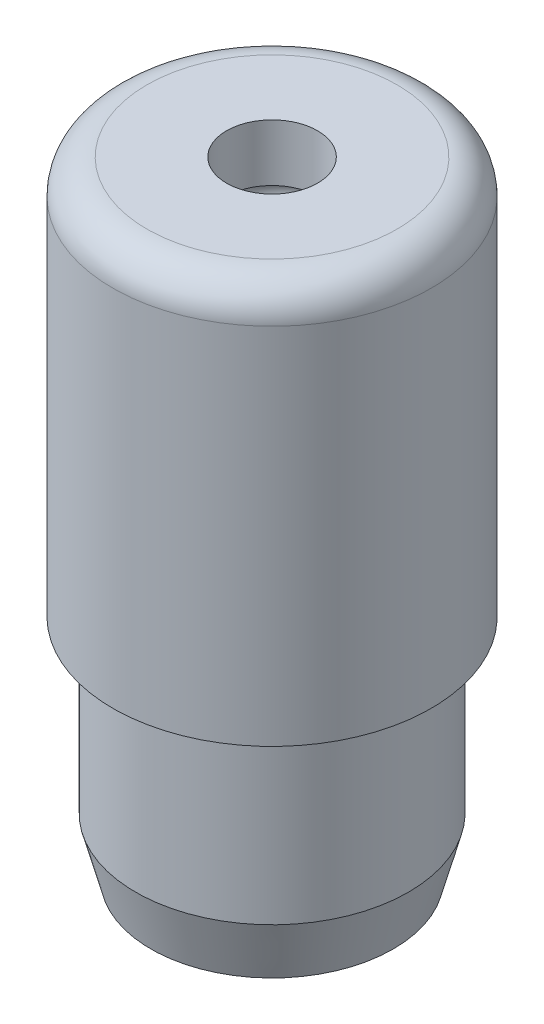
ISO-10303-21;
HEADER;
FILE_DESCRIPTION(('STEP AP214'),'2;1');
FILE_NAME('part.step','',(''),(''),'','','');
FILE_SCHEMA(('AUTOMOTIVE_DESIGN { 1 0 10303 214 1 1 1 1 }'));
ENDSEC;
DATA;
#1=APPLICATION_CONTEXT('core data for automotive mechanical design processes');
#2=APPLICATION_PROTOCOL_DEFINITION('international standard','automotive_design',2000,#1);
#3=PRODUCT_CONTEXT('',#1,'mechanical');
#4=PRODUCT('Part','Part','',(#3));
#5=PRODUCT_RELATED_PRODUCT_CATEGORY('part','',(#4));
#6=PRODUCT_DEFINITION_FORMATION('','',#4);
#7=PRODUCT_DEFINITION_CONTEXT('part definition',#1,'design');
#8=PRODUCT_DEFINITION('design','',#6,#7);
#9=PRODUCT_DEFINITION_SHAPE('','',#8);
#10=(LENGTH_UNIT() NAMED_UNIT(*) SI_UNIT(.MILLI.,.METRE.));
#11=(NAMED_UNIT(*) PLANE_ANGLE_UNIT() SI_UNIT($,.RADIAN.));
#12=(NAMED_UNIT(*) SI_UNIT($,.STERADIAN.) SOLID_ANGLE_UNIT());
#13=UNCERTAINTY_MEASURE_WITH_UNIT(LENGTH_MEASURE(1.E-05),#10,'distance_accuracy_value','');
#14=(GEOMETRIC_REPRESENTATION_CONTEXT(3) GLOBAL_UNCERTAINTY_ASSIGNED_CONTEXT((#13)) GLOBAL_UNIT_ASSIGNED_CONTEXT((#10,
#11,#12)) REPRESENTATION_CONTEXT('',''));
#15=CARTESIAN_POINT('',(0.,0.,0.));
#16=DIRECTION('',(0.,0.,1.));
#17=DIRECTION('',(1.,0.,0.));
#18=AXIS2_PLACEMENT_3D('',#15,#16,#17);
#19=CARTESIAN_POINT('',(0.,148.45149792253,0.));
#20=DIRECTION('',(0.,1.,0.));
#21=DIRECTION('',(-1.,0.,0.));
#22=AXIS2_PLACEMENT_3D('',#19,#20,#21);
#23=CYLINDRICAL_SURFACE('',#22,12.);
#24=CARTESIAN_POINT('',(0.,15.1898640484145,0.));
#25=DIRECTION('',(0.,1.,0.));
#26=DIRECTION('',(-1.,0.,0.));
#27=AXIS2_PLACEMENT_3D('',#24,#25,#26);
#28=CIRCLE('',#27,12.);
#29=CARTESIAN_POINT('',(-12.,15.1898640484145,0.));
#30=VERTEX_POINT('',#29);
#31=EDGE_CURVE('E81',#30,#30,#28,.T.);
#32=ORIENTED_EDGE('',*,*,#31,.T.);
#33=EDGE_LOOP('',(#32));
#34=FACE_BOUND('',#33,.T.);
#35=CARTESIAN_POINT('',(0.,30.1898640484145,0.));
#36=DIRECTION('',(0.,1.,0.));
#37=DIRECTION('',(-1.,0.,0.));
#38=AXIS2_PLACEMENT_3D('',#35,#36,#37);
#39=CIRCLE('',#38,12.);
#40=CARTESIAN_POINT('',(-12.,30.1898640484145,0.));
#41=VERTEX_POINT('',#40);
#42=EDGE_CURVE('E10',#41,#41,#39,.T.);
#43=ORIENTED_EDGE('',*,*,#42,.F.);
#44=EDGE_LOOP('',(#43));
#45=FACE_BOUND('',#44,.T.);
#46=ADVANCED_FACE('F40',(#34,#45),#23,.T.);
#47=CARTESIAN_POINT('',(-14.,30.1898640484145,0.));
#48=DIRECTION('',(0.,-1.,0.));
#49=DIRECTION('',(1.,0.,0.));
#50=AXIS2_PLACEMENT_3D('',#47,#48,#49);
#51=PLANE('',#50);
#52=ORIENTED_EDGE('',*,*,#42,.T.);
#53=EDGE_LOOP('',(#52));
#54=FACE_BOUND('',#53,.T.);
#55=CARTESIAN_POINT('',(0.,30.1898640484145,0.));
#56=DIRECTION('',(0.,1.,0.));
#57=DIRECTION('',(-1.,0.,0.));
#58=AXIS2_PLACEMENT_3D('',#55,#56,#57);
#59=CIRCLE('',#58,14.);
#60=CARTESIAN_POINT('',(-14.,30.1898640484145,0.));
#61=VERTEX_POINT('',#60);
#62=EDGE_CURVE('E43',#61,#61,#59,.T.);
#63=ORIENTED_EDGE('',*,*,#62,.F.);
#64=EDGE_LOOP('',(#63));
#65=FACE_BOUND('',#64,.T.);
#66=ADVANCED_FACE('F102',(#54,#65),#51,.T.);
#67=CARTESIAN_POINT('',(0.,148.45149792253,0.));
#68=DIRECTION('',(0.,1.,0.));
#69=DIRECTION('',(-1.,0.,0.));
#70=AXIS2_PLACEMENT_3D('',#67,#68,#69);
#71=CYLINDRICAL_SURFACE('',#70,14.);
#72=ORIENTED_EDGE('',*,*,#62,.T.);
#73=EDGE_LOOP('',(#72));
#74=FACE_BOUND('',#73,.T.);
#75=CARTESIAN_POINT('',(0.,62.1898640484145,0.));
#76=DIRECTION('',(0.,1.,0.));
#77=DIRECTION('',(-1.,0.,0.));
#78=AXIS2_PLACEMENT_3D('',#75,#76,#77);
#79=CIRCLE('',#78,14.);
#80=CARTESIAN_POINT('',(-14.,62.1898640484145,0.));
#81=VERTEX_POINT('',#80);
#82=EDGE_CURVE('E50',#81,#81,#79,.T.);
#83=ORIENTED_EDGE('',*,*,#82,.F.);
#84=EDGE_LOOP('',(#83));
#85=FACE_BOUND('',#84,.T.);
#86=ADVANCED_FACE('F103',(#74,#85),#71,.T.);
#87=CARTESIAN_POINT('',(0.,62.1898640484145,0.));
#88=DIRECTION('',(0.,1.,0.));
#89=DIRECTION('',(-1.,0.,0.));
#90=AXIS2_PLACEMENT_3D('',#87,#88,#89);
#91=TOROIDAL_SURFACE('',#90,11.,3.);
#92=ORIENTED_EDGE('',*,*,#82,.T.);
#93=EDGE_LOOP('',(#92));
#94=FACE_BOUND('',#93,.T.);
#95=CARTESIAN_POINT('',(0.,65.1898640484145,0.));
#96=DIRECTION('',(0.,1.,0.));
#97=DIRECTION('',(-1.,0.,0.));
#98=AXIS2_PLACEMENT_3D('',#95,#96,#97);
#99=CIRCLE('',#98,11.);
#100=CARTESIAN_POINT('',(-11.,65.1898640484145,0.));
#101=VERTEX_POINT('',#100);
#102=EDGE_CURVE('E51',#101,#101,#99,.T.);
#103=ORIENTED_EDGE('',*,*,#102,.F.);
#104=EDGE_LOOP('',(#103));
#105=FACE_BOUND('',#104,.T.);
#106=ADVANCED_FACE('F109',(#94,#105),#91,.T.);
#107=CARTESIAN_POINT('',(-4.0000000000018,65.1898640484145,0.));
#108=DIRECTION('',(0.,1.,0.));
#109=DIRECTION('',(-1.,0.,0.));
#110=AXIS2_PLACEMENT_3D('',#107,#108,#109);
#111=PLANE('',#110);
#112=ORIENTED_EDGE('',*,*,#102,.T.);
#113=EDGE_LOOP('',(#112));
#114=FACE_BOUND('',#113,.T.);
#115=CARTESIAN_POINT('',(0.,65.1898640484145,0.));
#116=DIRECTION('',(0.,1.,0.));
#117=DIRECTION('',(-1.,0.,0.));
#118=AXIS2_PLACEMENT_3D('',#115,#116,#117);
#119=CIRCLE('',#118,4.00000000000181);
#120=CARTESIAN_POINT('',(-4.0000000000018,65.1898640484145,0.));
#121=VERTEX_POINT('',#120);
#122=EDGE_CURVE('E57',#121,#121,#119,.T.);
#123=ORIENTED_EDGE('',*,*,#122,.F.);
#124=EDGE_LOOP('',(#123));
#125=FACE_BOUND('',#124,.T.);
#126=ADVANCED_FACE('F113',(#114,#125),#111,.T.);
#127=CARTESIAN_POINT('',(0.,148.45149792253,0.));
#128=DIRECTION('',(0.,1.,0.));
#129=DIRECTION('',(-1.,0.,0.));
#130=AXIS2_PLACEMENT_3D('',#127,#128,#129);
#131=CYLINDRICAL_SURFACE('',#130,4.00000000000181);
#132=ORIENTED_EDGE('',*,*,#122,.T.);
#133=EDGE_LOOP('',(#132));
#134=FACE_BOUND('',#133,.T.);
#135=CARTESIAN_POINT('',(0.,60.1898640484145,0.));
#136=DIRECTION('',(0.,1.,0.));
#137=DIRECTION('',(-1.,0.,0.));
#138=AXIS2_PLACEMENT_3D('',#135,#136,#137);
#139=CIRCLE('',#138,4.00000000000181);
#140=CARTESIAN_POINT('',(-4.0000000000018,60.1898640484145,0.));
#141=VERTEX_POINT('',#140);
#142=EDGE_CURVE('E56',#141,#141,#139,.T.);
#143=ORIENTED_EDGE('',*,*,#142,.F.);
#144=EDGE_LOOP('',(#143));
#145=FACE_BOUND('',#144,.T.);
#146=ADVANCED_FACE('F119',(#134,#145),#131,.F.);
#147=CARTESIAN_POINT('',(0.,58.6898640484145,0.));
#148=DIRECTION('',(0.,1.,0.));
#149=DIRECTION('',(-1.,0.,0.));
#150=AXIS2_PLACEMENT_3D('',#147,#148,#149);
#151=TOROIDAL_SURFACE('',#150,3.99999999999999,1.5);
#152=ORIENTED_EDGE('',*,*,#142,.T.);
#153=EDGE_LOOP('',(#152));
#154=FACE_BOUND('',#153,.T.);
#155=CARTESIAN_POINT('',(0.,57.1898640484145,0.));
#156=DIRECTION('',(0.,1.,0.));
#157=DIRECTION('',(-1.,0.,0.));
#158=AXIS2_PLACEMENT_3D('',#155,#156,#157);
#159=CIRCLE('',#158,3.99999999999896);
#160=CARTESIAN_POINT('',(-3.99999999999895,57.1898640484145,0.));
#161=VERTEX_POINT('',#160);
#162=EDGE_CURVE('E65',#161,#161,#159,.T.);
#163=ORIENTED_EDGE('',*,*,#162,.F.);
#164=EDGE_LOOP('',(#163));
#165=FACE_BOUND('',#164,.T.);
#166=ADVANCED_FACE('F121',(#154,#165),#151,.F.);
#167=CARTESIAN_POINT('',(0.,148.45149792253,0.));
#168=DIRECTION('',(0.,1.,0.));
#169=DIRECTION('',(-1.,0.,0.));
#170=AXIS2_PLACEMENT_3D('',#167,#168,#169);
#171=CYLINDRICAL_SURFACE('',#170,3.99999999999947);
#172=ORIENTED_EDGE('',*,*,#162,.T.);
#173=EDGE_LOOP('',(#172));
#174=FACE_BOUND('',#173,.T.);
#175=CARTESIAN_POINT('',(0.,50.1898640484145,0.));
#176=DIRECTION('',(0.,1.,0.));
#177=DIRECTION('',(-1.,0.,0.));
#178=AXIS2_PLACEMENT_3D('',#175,#176,#177);
#179=CIRCLE('',#178,3.99999999999999);
#180=CARTESIAN_POINT('',(-3.99999999999998,50.1898640484145,0.));
#181=VERTEX_POINT('',#180);
#182=EDGE_CURVE('E61',#181,#181,#179,.T.);
#183=ORIENTED_EDGE('',*,*,#182,.F.);
#184=EDGE_LOOP('',(#183));
#185=FACE_BOUND('',#184,.T.);
#186=ADVANCED_FACE('F130',(#174,#185),#171,.F.);
#187=CARTESIAN_POINT('',(0.,48.6898640484145,0.));
#188=DIRECTION('',(0.,1.,0.));
#189=DIRECTION('',(-1.,0.,0.));
#190=AXIS2_PLACEMENT_3D('',#187,#188,#189);
#191=TOROIDAL_SURFACE('',#190,3.99999999999999,1.5);
#192=ORIENTED_EDGE('',*,*,#182,.T.);
#193=EDGE_LOOP('',(#192));
#194=FACE_BOUND('',#193,.T.);
#195=CARTESIAN_POINT('',(0.,47.1898640484145,0.));
#196=DIRECTION('',(0.,1.,0.));
#197=DIRECTION('',(-1.,0.,0.));
#198=AXIS2_PLACEMENT_3D('',#195,#196,#197);
#199=CIRCLE('',#198,3.99999999999999);
#200=CARTESIAN_POINT('',(-3.99999999999998,47.1898640484145,0.));
#201=VERTEX_POINT('',#200);
#202=EDGE_CURVE('E66',#201,#201,#199,.T.);
#203=ORIENTED_EDGE('',*,*,#202,.F.);
#204=EDGE_LOOP('',(#203));
#205=FACE_BOUND('',#204,.T.);
#206=ADVANCED_FACE('F131',(#194,#205),#191,.F.);
#207=CARTESIAN_POINT('',(0.,148.45149792253,0.));
#208=DIRECTION('',(0.,1.,0.));
#209=DIRECTION('',(-1.,0.,0.));
#210=AXIS2_PLACEMENT_3D('',#207,#208,#209);
#211=CYLINDRICAL_SURFACE('',#210,3.99999999999999);
#212=ORIENTED_EDGE('',*,*,#202,.T.);
#213=EDGE_LOOP('',(#212));
#214=FACE_BOUND('',#213,.T.);
#215=CARTESIAN_POINT('',(0.,38.1898640484145,0.));
#216=DIRECTION('',(0.,1.,0.));
#217=DIRECTION('',(-1.,0.,0.));
#218=AXIS2_PLACEMENT_3D('',#215,#216,#217);
#219=CIRCLE('',#218,3.99999999999999);
#220=CARTESIAN_POINT('',(-3.99999999999998,38.1898640484145,0.));
#221=VERTEX_POINT('',#220);
#222=EDGE_CURVE('E72',#221,#221,#219,.T.);
#223=ORIENTED_EDGE('',*,*,#222,.F.);
#224=EDGE_LOOP('',(#223));
#225=FACE_BOUND('',#224,.T.);
#226=ADVANCED_FACE('F134',(#214,#225),#211,.F.);
#227=CARTESIAN_POINT('',(0.,37.1898640484145,0.));
#228=DIRECTION('',(0.,-1.,0.));
#229=DIRECTION('',(1.,0.,0.));
#230=AXIS2_PLACEMENT_3D('',#227,#228,#229);
#231=CONICAL_SURFACE('',#230,5.,0.78539816339745);
#232=ORIENTED_EDGE('',*,*,#222,.T.);
#233=EDGE_LOOP('',(#232));
#234=FACE_BOUND('',#233,.T.);
#235=CARTESIAN_POINT('',(0.,37.1898640484145,0.));
#236=DIRECTION('',(0.,1.,0.));
#237=DIRECTION('',(-1.,0.,0.));
#238=AXIS2_PLACEMENT_3D('',#235,#236,#237);
#239=CIRCLE('',#238,5.);
#240=CARTESIAN_POINT('',(-4.99999999999998,37.1898640484145,0.));
#241=VERTEX_POINT('',#240);
#242=EDGE_CURVE('E74',#241,#241,#239,.T.);
#243=ORIENTED_EDGE('',*,*,#242,.F.);
#244=EDGE_LOOP('',(#243));
#245=FACE_BOUND('',#244,.T.);
#246=ADVANCED_FACE('F137',(#234,#245),#231,.F.);
#247=CARTESIAN_POINT('',(0.,148.45149792253,0.));
#248=DIRECTION('',(0.,1.,0.));
#249=DIRECTION('',(-1.,0.,0.));
#250=AXIS2_PLACEMENT_3D('',#247,#248,#249);
#251=CYLINDRICAL_SURFACE('',#250,5.);
#252=ORIENTED_EDGE('',*,*,#242,.T.);
#253=EDGE_LOOP('',(#252));
#254=FACE_BOUND('',#253,.T.);
#255=CARTESIAN_POINT('',(0.,10.1898640484145,0.));
#256=DIRECTION('',(0.,1.,0.));
#257=DIRECTION('',(-1.,0.,0.));
#258=AXIS2_PLACEMENT_3D('',#255,#256,#257);
#259=CIRCLE('',#258,5.);
#260=CARTESIAN_POINT('',(-4.99999999999998,10.1898640484145,0.));
#261=VERTEX_POINT('',#260);
#262=EDGE_CURVE('E77',#261,#261,#259,.T.);
#263=ORIENTED_EDGE('',*,*,#262,.F.);
#264=EDGE_LOOP('',(#263));
#265=FACE_BOUND('',#264,.T.);
#266=ADVANCED_FACE('F100',(#254,#265),#251,.F.);
#267=CARTESIAN_POINT('',(-10.6602540378444,10.1898640484145,0.));
#268=DIRECTION('',(0.,-1.,0.));
#269=DIRECTION('',(1.,0.,0.));
#270=AXIS2_PLACEMENT_3D('',#267,#268,#269);
#271=PLANE('',#270);
#272=ORIENTED_EDGE('',*,*,#262,.T.);
#273=EDGE_LOOP('',(#272));
#274=FACE_BOUND('',#273,.T.);
#275=CARTESIAN_POINT('',(0.,10.1898640484145,0.));
#276=DIRECTION('',(0.,1.,0.));
#277=DIRECTION('',(-1.,0.,0.));
#278=AXIS2_PLACEMENT_3D('',#275,#276,#277);
#279=CIRCLE('',#278,10.6602540378444);
#280=CARTESIAN_POINT('',(-10.6602540378444,10.1898640484145,0.));
#281=VERTEX_POINT('',#280);
#282=EDGE_CURVE('E79',#281,#281,#279,.T.);
#283=ORIENTED_EDGE('',*,*,#282,.F.);
#284=EDGE_LOOP('',(#283));
#285=FACE_BOUND('',#284,.T.);
#286=ADVANCED_FACE('F91',(#274,#285),#271,.T.);
#287=CARTESIAN_POINT('',(0.,15.1898640484145,0.));
#288=DIRECTION('',(0.,1.,0.));
#289=DIRECTION('',(-1.,0.,0.));
#290=AXIS2_PLACEMENT_3D('',#287,#288,#289);
#291=CONICAL_SURFACE('',#290,12.,0.261799387799151);
#292=ORIENTED_EDGE('',*,*,#282,.T.);
#293=EDGE_LOOP('',(#292));
#294=FACE_BOUND('',#293,.T.);
#295=ORIENTED_EDGE('',*,*,#31,.F.);
#296=EDGE_LOOP('',(#295));
#297=FACE_BOUND('',#296,.T.);
#298=ADVANCED_FACE('F87',(#294,#297),#291,.T.);
#299=CLOSED_SHELL('',(#46,#66,#86,#106,#126,#146,#166,#186,#206,#226,#246,#266,#286,#298));
#300=MANIFOLD_SOLID_BREP('B2',#299);
#301=ADVANCED_BREP_SHAPE_REPRESENTATION('',(#18,#300),#14);
#302=SHAPE_DEFINITION_REPRESENTATION(#9,#301);
ENDSEC;
END-ISO-10303-21;
